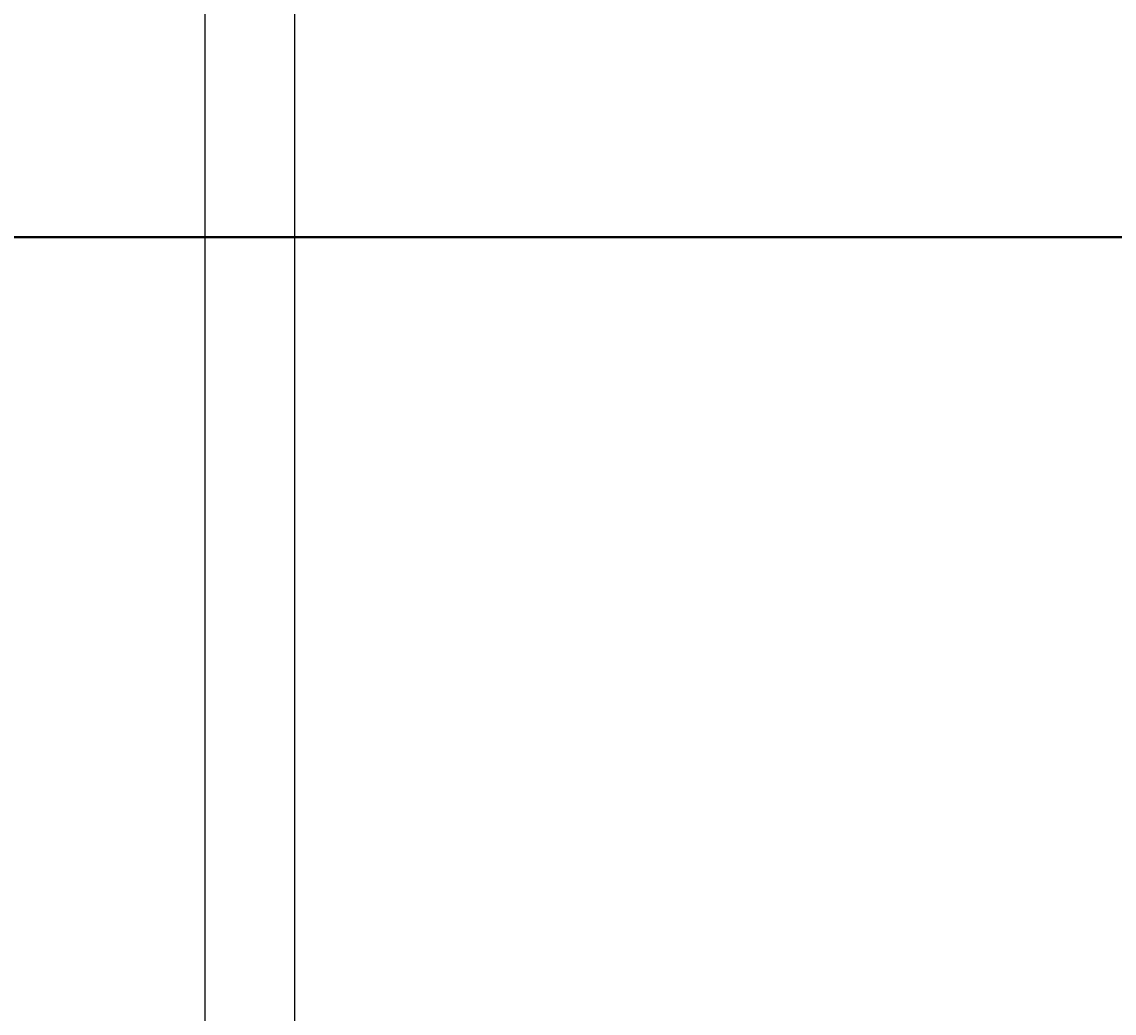
# Model space of a CAD drawing. Units: inches. Extents: x -6 to 289, y -8 to 323.
# Tile 93 of 107: x 196 to 222, y 229 to 252. Entities that reach past the tile are written whole.
import ezdxf

# ---------------------------------------------------------------- set-up
doc = ezdxf.new("R2010")
doc.units = ezdxf.units.IN
doc.header["$MEASUREMENT"] = 0
doc.layers.add('A-ANNO-DIMS', color=2, linetype='Continuous', lineweight=18)
doc.layers.add('A-ELEV', color=7, linetype='Continuous', lineweight=35)
doc.styles.get("Standard").update_dxf_attribs({"font": 'arial.ttf'})
doc.dimstyles.get("Standard").update_dxf_attribs({"dimtxt": 0.18, "dimasz": 0.18, "dimexe": 0.18, "dimexo": 0.0625, "dimgap": 0.09, "dimtad": 0, "dimtih": 1, "dimtoh": 1, "dimdec": 4, "dimzin": 0, "dimdsep": 46, "dimtxsty": 'Standard', "dimcen": 0.09, "dimadec": 0, "dimazin": 0, "dimtfac": 1, "dimtdec": 4, "dimtofl": 0, "dimtmove": 0, "dimatfit": 3, "dimfxl": 1, "dimtolj": 1, "dimtzin": 0, "dimarcsym": 0})

# ---------------------------------------------------------------- blocks, each defined once
blk = doc.blocks.new('*D13')
at = {"layer": 'A-ANNO-DIMS', "color": 0, "lineweight": -2, "transparency": 16777216}
for p, q in [((188.292, 226.951), (188.292, 322.969)), ((236.292, 226.951), (236.292, 322.969)), ((188.472, 322.789), (212.069, 322.789)), ((236.112, 322.789), (212.515, 322.789))]:
    blk.add_line(p, q, dxfattribs=at)
at = {"layer": 'A-ANNO-DIMS', "color": 0, "transparency": 16777216}
for points in [[(188.472, 322.819), (188.472, 322.759), (188.292, 322.789)], [(236.112, 322.819), (236.112, 322.759), (236.292, 322.789)]]:
    blk.add_solid(points, dxfattribs=at)
at = {"layer": 'Defpoints', "color": 0, "transparency": 16777216}
for p in [(236.292, 322.789), (188.292, 226.889), (236.292, 226.889)]:
    blk.add_point(p, dxfattribs=at)
at = {"layer": 'A-ANNO-DIMS', "color": 0, "transparency": 16777216, "insert": (212.292, 322.789), "char_height": 0.18, "attachment_point": 5}
blk.add_mtext('\\A1;48', dxfattribs=at)
blk = doc.blocks.new('*D26')
at = {"layer": 'A-ANNO-DIMS', "color": 0, "lineweight": -2, "transparency": 16777216}
for p, q in [((247.226, 247.289), (288.653, 247.289)), ((288.473, 247.109), (288.473, 237.153)), ((288.473, 226.834), (288.473, 236.789)), ((126.946, 226.654), (288.653, 226.654))]:
    blk.add_line(p, q, dxfattribs=at)
at = {"layer": 'A-ANNO-DIMS', "color": 0, "transparency": 16777216}
for points in [[(288.443, 247.109), (288.503, 247.109), (288.473, 247.289)], [(288.443, 226.834), (288.503, 226.834), (288.473, 226.654)]]:
    blk.add_solid(points, dxfattribs=at)
at = {"layer": 'Defpoints', "color": 0, "transparency": 16777216}
for p in [(247.164, 247.289), (288.473, 247.289), (126.883, 226.654)]:
    blk.add_point(p, dxfattribs=at)
at = {"layer": 'A-ANNO-DIMS', "color": 0, "transparency": 16777216, "insert": (288.473, 236.971), "char_height": 0.18, "attachment_point": 5}
blk.add_mtext('\\A1;20.635', dxfattribs=at)
blk = doc.blocks.new('*D27')
at = {"layer": 'A-ANNO-DIMS', "color": 0, "lineweight": -2, "transparency": 16777216}
for p, q in [((19.226, 307.289), (288.653, 307.289)), ((288.473, 307.109), (288.473, 277.471)), ((288.473, 247.469), (288.473, 277.107)), ((247.226, 247.289), (288.653, 247.289))]:
    blk.add_line(p, q, dxfattribs=at)
at = {"layer": 'A-ANNO-DIMS', "color": 0, "transparency": 16777216}
for points in [[(288.443, 307.109), (288.503, 307.109), (288.473, 307.289)], [(288.443, 247.469), (288.503, 247.469), (288.473, 247.289)]]:
    blk.add_solid(points, dxfattribs=at)
at = {"layer": 'Defpoints', "color": 0, "transparency": 16777216}
for p in [(19.164, 307.289), (288.473, 307.289), (247.164, 247.289)]:
    blk.add_point(p, dxfattribs=at)
at = {"layer": 'A-ANNO-DIMS', "color": 0, "transparency": 16777216, "insert": (288.473, 277.289), "char_height": 0.18, "attachment_point": 5}
blk.add_mtext('\\A1;60', dxfattribs=at)
blk = doc.blocks.new('*D80')
at = {"layer": 'A-ANNO-DIMS', "color": 0, "lineweight": -2, "transparency": 16777216}
for p, q in [((188.292, 116.842), (188.292, 322.969)), ((230.292, 116.842), (230.292, 322.969)), ((188.472, 322.789), (209.07, 322.789)), ((230.112, 322.789), (209.513, 322.789))]:
    blk.add_line(p, q, dxfattribs=at)
at = {"layer": 'A-ANNO-DIMS', "color": 0, "transparency": 16777216}
for points in [[(188.472, 322.819), (188.472, 322.759), (188.292, 322.789)], [(230.112, 322.819), (230.112, 322.759), (230.292, 322.789)]]:
    blk.add_solid(points, dxfattribs=at)
at = {"layer": 'Defpoints', "color": 0, "transparency": 16777216}
for p in [(230.292, 322.789), (188.292, 116.779), (230.292, 116.779)]:
    blk.add_point(p, dxfattribs=at)
at = {"layer": 'A-ANNO-DIMS', "color": 0, "transparency": 16777216, "insert": (209.292, 322.789), "char_height": 0.18, "attachment_point": 5}
blk.add_mtext('\\A1;42', dxfattribs=at)
blk = doc.blocks.new('*D96')
at = {"layer": 'A-ANNO-DIMS', "color": 0, "lineweight": -2, "transparency": 16777216}
for p, q in [((164.004, 159.411), (164.004, 322.969)), ((200.616, 159.411), (200.616, 322.969)), ((164.184, 322.789), (181.934, 322.789)), ((200.436, 322.789), (182.686, 322.789))]:
    blk.add_line(p, q, dxfattribs=at)
at = {"layer": 'A-ANNO-DIMS', "color": 0, "transparency": 16777216}
for points in [[(164.184, 322.819), (164.184, 322.759), (164.004, 322.789)], [(200.436, 322.819), (200.436, 322.759), (200.616, 322.789)]]:
    blk.add_solid(points, dxfattribs=at)
at = {"layer": 'Defpoints', "color": 0, "transparency": 16777216}
for p in [(200.616, 322.789), (164.004, 159.348), (200.616, 159.348)]:
    blk.add_point(p, dxfattribs=at)
at = {"layer": 'A-ANNO-DIMS', "color": 0, "transparency": 16777216, "insert": (182.31, 322.789), "char_height": 0.18, "attachment_point": 5}
blk.add_mtext('\\A1;36.61', dxfattribs=at)
blk = doc.blocks.new('*D97')
at = {"layer": 'A-ANNO-DIMS', "color": 0, "lineweight": -2, "transparency": 16777216}
for p, q in [((200.616, 159.411), (200.616, 322.969)), ((202.741, 159.411), (202.741, 322.969)), ((200.796, 322.789), (201.283, 322.789)), ((202.561, 322.789), (202.075, 322.789))]:
    blk.add_line(p, q, dxfattribs=at)
at = {"layer": 'A-ANNO-DIMS', "color": 0, "transparency": 16777216}
for points in [[(200.796, 322.819), (200.796, 322.759), (200.616, 322.789)], [(202.561, 322.819), (202.561, 322.759), (202.741, 322.789)]]:
    blk.add_solid(points, dxfattribs=at)
at = {"layer": 'Defpoints', "color": 0, "transparency": 16777216}
for p in [(202.741, 322.789), (200.616, 159.348), (202.741, 159.348)]:
    blk.add_point(p, dxfattribs=at)
at = {"layer": 'A-ANNO-DIMS', "color": 0, "transparency": 16777216, "insert": (201.679, 322.789), "char_height": 0.18, "attachment_point": 5}
blk.add_mtext('\\A1;2.125', dxfattribs=at)
blk = doc.blocks.new('*D98')
at = {"layer": 'A-ANNO-DIMS', "color": 0, "lineweight": -2, "transparency": 16777216}
for p, q in [((202.741, 159.411), (202.741, 322.969)), ((244.164, 159.411), (244.164, 322.969)), ((202.921, 322.789), (223.056, 322.789)), ((243.984, 322.789), (223.849, 322.789))]:
    blk.add_line(p, q, dxfattribs=at)
at = {"layer": 'A-ANNO-DIMS', "color": 0, "transparency": 16777216}
for points in [[(202.921, 322.819), (202.921, 322.759), (202.741, 322.789)], [(243.984, 322.819), (243.984, 322.759), (244.164, 322.789)]]:
    blk.add_solid(points, dxfattribs=at)
at = {"layer": 'Defpoints', "color": 0, "transparency": 16777216}
for p in [(244.164, 322.789), (202.741, 159.348), (244.164, 159.348)]:
    blk.add_point(p, dxfattribs=at)
at = {"layer": 'A-ANNO-DIMS', "color": 0, "transparency": 16777216, "insert": (223.452, 322.789), "char_height": 0.18, "attachment_point": 5}
blk.add_mtext('\\A1;41.42', dxfattribs=at)

msp = doc.modelspace()

# ---------------------------------------------------------------- linework, layer by layer
at = {"layer": 'A-ELEV'}
for p, q in [((247.1638, 247.2888), (115.1638, 247.2888)), ((115.1638, 247.2888), (247.1638, 247.2888))]:
    msp.add_line(p, q, dxfattribs=at)

# ---------------------------------------------------------------- dimensions: what is measured, and where the dimension line sits
at = {"layer": 'A-ANNO-DIMS'}
for base, p1, p2, override, picture, middle in [((200.6162, 322.7888), (164.0039, 159.3484), (200.6162, 159.3484), {"dimdec": 2, "dimlfac": 1, "dimrnd": 0, "dimzin": 0, "dimdsep": 46, "dimlunit": 2}, '*D96', (182.3101, 322.7888)), ((236.2918, 322.7888), (188.2918, 226.8887), (236.2918, 226.8887), {"dimdec": 0, "dimlfac": 1, "dimrnd": 0, "dimzin": 0, "dimdsep": 46, "dimlunit": 2}, '*D13', (212.2918, 322.7888)), ((230.2918, 322.7888), (188.2918, 116.7795), (230.2918, 116.7795), {"dimdec": 0, "dimlfac": 1, "dimrnd": 0, "dimzin": 0, "dimdsep": 46, "dimlunit": 2}, '*D80', (209.2918, 322.7888)), ((202.741, 322.7888), (200.6162, 159.3484), (202.741, 159.3484), {"dimdec": 3, "dimlfac": 1, "dimrnd": 0, "dimzin": 0, "dimdsep": 46, "dimlunit": 2}, '*D97', (201.6786, 322.7888)), ((244.1638, 322.7888), (202.741, 159.3484), (244.1638, 159.3484), {"dimdec": 2, "dimlfac": 1, "dimrnd": 0, "dimzin": 0, "dimdsep": 46, "dimlunit": 2}, '*D98', (223.4524, 322.7888))]:
    dim = msp.add_linear_dim(base=base, p1=p1, p2=p2, dimstyle='Standard', override=override, dxfattribs=at)
    dim.commit()
    dim.dimension.update_dxf_attribs({"geometry": picture, "text_midpoint": middle})
for base, p1, p2, override, picture, middle in [((288.4733, 307.2888), (247.1638, 247.2888), (19.1638, 307.2888), {"dimdec": 0, "dimlfac": 1, "dimrnd": 0, "dimzin": 0, "dimdsep": 46, "dimlunit": 2}, '*D27', (288.4733, 277.2888)), ((288.4733, 247.2888), (126.8835, 226.654), (247.1638, 247.2888), {"dimdec": 3, "dimlfac": 1, "dimrnd": 0, "dimzin": 0, "dimdsep": 46, "dimlunit": 2}, '*D26', (288.4733, 236.9714))]:
    dim = msp.add_linear_dim(base=base, p1=p1, p2=p2, angle=90, dimstyle='Standard', override=override, dxfattribs=at)
    dim.commit()
    dim.dimension.update_dxf_attribs({"geometry": picture, "text_midpoint": middle})

doc.saveas('drawing.dxf')
